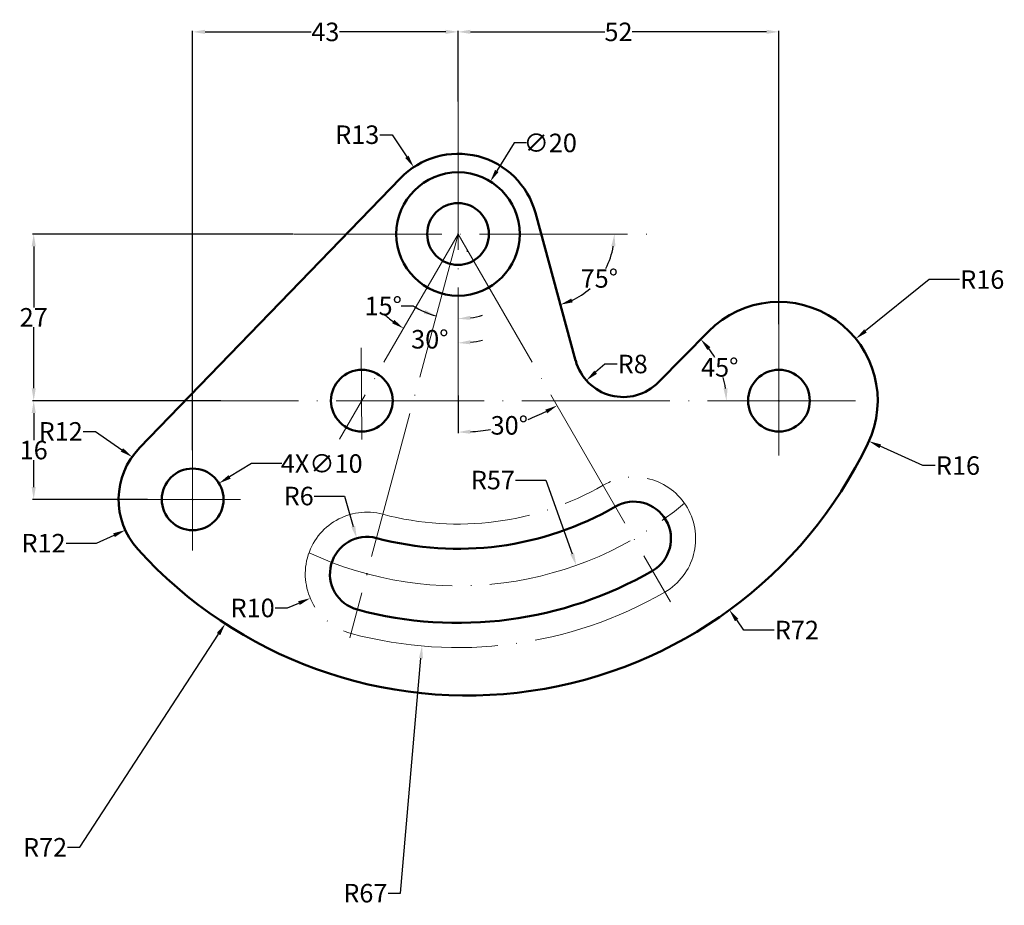
# Model space of a CAD drawing. Units: inches. Extents: x 244 to 404, y 121 to 265.
import ezdxf

# ---------------------------------------------------------------- set-up
doc = ezdxf.new("R2010")
doc.units = ezdxf.units.IN
doc.header["$MEASUREMENT"] = 0
doc.linetypes.add('ACAD_ISO04W100', pattern=[30, 24, -3, 0, -3])
for name, color, linetype, lineweight in [('M-CNTR', 4, 'ACAD_ISO04W100', 18), ('M-CONS', 4, 'ACAD_ISO04W100', 18), ('M-DIMS', 2, 'Continuous', 25), ('M-OUTL', 7, 'Continuous', 50)]:
    doc.layers.add(name, color=color, linetype=linetype, lineweight=lineweight)
doc.styles.get("Standard").update_dxf_attribs({"font": 'arial.ttf'})
doc.dimstyles.get("Standard").update_dxf_attribs({"dimtxt": 3, "dimasz": 2, "dimexe": 0.18, "dimexo": 0.0625, "dimgap": 0.09, "dimtad": 0, "dimtih": 1, "dimtoh": 1, "dimdec": 0, "dimzin": 0, "dimdsep": 46, "dimtxsty": 'Standard', "dimcen": 0.09, "dimadec": 0, "dimazin": 0, "dimtfac": 1, "dimtdec": 0, "dimtofl": 0, "dimtmove": 0, "dimatfit": 3, "dimfxl": 1, "dimtolj": 1, "dimtzin": 0, "dimarcsym": 0})

# ---------------------------------------------------------------- blocks, each defined once
blk = doc.blocks.new('*D1')
at = {"layer": 'Defpoints', "color": 0, "transparency": 16777216}
for p in [(316.73, 227.26), (359.19, 169.11)]:
    blk.add_point(p, dxfattribs=at)
at = {"layer": 'M-DIMS', "color": 0, "lineweight": -2, "transparency": 16777216}
for p, q in [((316.64, 227.26), (316.82, 227.26)), ((316.73, 227.17), (316.73, 227.35)), ((361.55, 165.87), (360.37, 167.5)), ((366.47, 165.87), (361.55, 165.87))]:
    blk.add_line(p, q, dxfattribs=at)
at = {"layer": 'M-DIMS', "color": 0, "transparency": 16777216}
blk.add_solid([(360.64, 167.69), (360.1, 167.3), (359.19, 169.11)], dxfattribs=at)
at = {"layer": 'M-DIMS', "color": 0, "transparency": 16777216, "insert": (370.13, 165.87), "char_height": 3, "attachment_point": 5}
blk.add_mtext('\\A1;R72', dxfattribs=at)
blk = doc.blocks.new('*D2')
at = {"layer": 'Defpoints', "color": 0, "transparency": 16777216}
for p in [(315.22, 230.03), (334.38, 176.35)]:
    blk.add_point(p, dxfattribs=at)
at = {"layer": 'M-DIMS', "color": 0, "lineweight": -2, "transparency": 16777216}
for p, q in [((324.54, 190.17), (329.45, 190.17)), ((329.45, 190.17), (333.71, 178.23))]:
    blk.add_line(p, q, dxfattribs=at)
at = {"layer": 'M-DIMS', "color": 0, "transparency": 16777216}
blk.add_solid([(334.02, 178.35), (333.4, 178.12), (334.38, 176.35)], dxfattribs=at)
at = {"layer": 'M-DIMS', "color": 0, "transparency": 16777216, "insert": (320.87, 190.17), "char_height": 3, "attachment_point": 5}
blk.add_mtext('\\A1;R57', dxfattribs=at)
blk = doc.blocks.new('*D3')
at = {"layer": 'Defpoints', "color": 0, "transparency": 16777216}
for p in [(300.47, 174.97), (291.28, 171.03)]:
    blk.add_point(p, dxfattribs=at)
at = {"layer": 'M-DIMS', "color": 0, "lineweight": -2, "transparency": 16777216}
for p, q in [((300.38, 174.97), (300.56, 174.97)), ((300.47, 174.88), (300.47, 175.06)), ((285.61, 169.45), (287.61, 169.45)), ((287.61, 169.45), (289.44, 170.24))]:
    blk.add_line(p, q, dxfattribs=at)
at = {"layer": 'M-DIMS', "color": 0, "transparency": 16777216}
blk.add_solid([(289.31, 170.54), (289.57, 169.93), (291.28, 171.03)], dxfattribs=at)
at = {"layer": 'M-DIMS', "color": 0, "transparency": 16777216, "insert": (281.94, 169.45), "char_height": 3, "attachment_point": 5}
blk.add_mtext('\\A1;R10', dxfattribs=at)
blk = doc.blocks.new('*D4')
at = {"layer": 'Defpoints', "color": 0, "transparency": 16777216}
for p in [(298.8, 180.74), (300.47, 174.97)]:
    blk.add_point(p, dxfattribs=at)
at = {"layer": 'M-DIMS', "color": 0, "lineweight": -2, "transparency": 16777216}
for p, q in [((291.91, 187.58), (296.81, 187.58)), ((296.81, 187.58), (298.24, 182.66)), ((300.38, 174.97), (300.56, 174.97)), ((300.47, 174.88), (300.47, 175.06))]:
    blk.add_line(p, q, dxfattribs=at)
at = {"layer": 'M-DIMS', "color": 0, "transparency": 16777216}
blk.add_solid([(298.56, 182.75), (297.92, 182.57), (298.8, 180.74)], dxfattribs=at)
at = {"layer": 'M-DIMS', "color": 0, "transparency": 16777216, "insert": (289.4, 187.58), "char_height": 3, "attachment_point": 5}
blk.add_mtext('\\A1;R6', dxfattribs=at)
blk = doc.blocks.new('*D5')
at = {"layer": 'Defpoints', "color": 0, "transparency": 16777216}
for p in [(272.22, 187.03), (261.3, 182.06)]:
    blk.add_point(p, dxfattribs=at)
at = {"layer": 'M-DIMS', "color": 0, "lineweight": -2, "transparency": 16777216}
for p, q in [((272.13, 187.03), (272.31, 187.03)), ((272.22, 186.94), (272.22, 187.12)), ((256.64, 179.94), (259.48, 181.23)), ((251.72, 179.94), (256.64, 179.94))]:
    blk.add_line(p, q, dxfattribs=at)
at = {"layer": 'M-DIMS', "color": 0, "transparency": 16777216}
blk.add_solid([(259.34, 181.54), (259.62, 180.93), (261.3, 182.06)], dxfattribs=at)
at = {"layer": 'M-DIMS', "color": 0, "transparency": 16777216, "insert": (248.06, 179.94), "char_height": 3, "attachment_point": 5}
blk.add_mtext('\\A1;R12', dxfattribs=at)
blk = doc.blocks.new('*D6')
at = {"layer": 'Defpoints', "color": 0, "transparency": 16777216}
for p in [(276.49, 189.64), (267.95, 184.43)]:
    blk.add_point(p, dxfattribs=at)
at = {"layer": 'M-DIMS', "color": 0, "lineweight": -2, "transparency": 16777216}
for p, q in [((281.73, 192.84), (278.2, 190.68)), ((286.65, 192.84), (281.73, 192.84)), ((272.13, 187.03), (272.31, 187.03)), ((272.22, 186.94), (272.22, 187.12))]:
    blk.add_line(p, q, dxfattribs=at)
at = {"layer": 'M-DIMS', "color": 0, "transparency": 16777216}
blk.add_solid([(278.02, 190.96), (278.37, 190.39), (276.49, 189.64)], dxfattribs=at)
at = {"layer": 'M-DIMS', "color": 0, "transparency": 16777216, "insert": (293.13, 192.84), "char_height": 3, "attachment_point": 5}
blk.add_mtext('\\A1;4X∅10', dxfattribs=at)
blk = doc.blocks.new('*D7')
at = {"layer": 'Defpoints', "color": 0, "transparency": 16777216}
for p in [(246.46, 203.03), (276.82, 203.03), (264.96, 187.03)]:
    blk.add_point(p, dxfattribs=at)
at = {"layer": 'M-DIMS', "color": 0, "lineweight": -2, "transparency": 16777216}
for p, q in [((276.76, 203.03), (246.28, 203.03)), ((246.46, 201.03), (246.46, 196.65)), ((246.46, 189.03), (246.46, 193.41)), ((264.89, 187.03), (246.28, 187.03))]:
    blk.add_line(p, q, dxfattribs=at)
at = {"layer": 'M-DIMS', "color": 0, "transparency": 16777216}
for points in [[(246.13, 201.03), (246.8, 201.03), (246.46, 203.03)], [(246.13, 189.03), (246.8, 189.03), (246.46, 187.03)]]:
    blk.add_solid(points, dxfattribs=at)
at = {"layer": 'M-DIMS', "color": 0, "transparency": 16777216, "insert": (246.46, 195.03), "char_height": 3, "attachment_point": 5}
blk.add_mtext('\\A1;16', dxfattribs=at)
blk = doc.blocks.new('*D8')
at = {"layer": 'Defpoints', "color": 0, "transparency": 16777216}
for p in [(246.46, 230.03), (288.6, 230.03), (276.82, 203.03)]:
    blk.add_point(p, dxfattribs=at)
at = {"layer": 'M-DIMS', "color": 0, "lineweight": -2, "transparency": 16777216}
for p, q in [((288.53, 230.03), (246.28, 230.03)), ((246.46, 228.03), (246.46, 218.13)), ((246.46, 205.03), (246.46, 214.94)), ((276.76, 203.03), (246.28, 203.03))]:
    blk.add_line(p, q, dxfattribs=at)
at = {"layer": 'M-DIMS', "color": 0, "transparency": 16777216}
for points in [[(246.13, 228.03), (246.8, 228.03), (246.46, 230.03)], [(246.13, 205.03), (246.8, 205.03), (246.46, 203.03)]]:
    blk.add_solid(points, dxfattribs=at)
at = {"layer": 'M-DIMS', "color": 0, "transparency": 16777216, "insert": (246.46, 216.53), "char_height": 3, "attachment_point": 5}
blk.add_mtext('\\A1;27', dxfattribs=at)
blk = doc.blocks.new('*D9')
at = {"layer": 'Defpoints', "color": 0, "transparency": 16777216}
for p in [(315.22, 262.78), (315.22, 251.46), (272.22, 194.96)]:
    blk.add_point(p, dxfattribs=at)
at = {"layer": 'M-DIMS', "color": 0, "lineweight": -2, "transparency": 16777216}
for p, q in [((272.22, 195.02), (272.22, 262.96)), ((274.22, 262.78), (291.42, 262.78)), ((313.22, 262.78), (296.02, 262.78)), ((315.22, 251.52), (315.22, 262.96))]:
    blk.add_line(p, q, dxfattribs=at)
at = {"layer": 'M-DIMS', "color": 0, "transparency": 16777216}
for points in [[(274.22, 263.12), (274.22, 262.45), (272.22, 262.78)], [(313.22, 263.12), (313.22, 262.45), (315.22, 262.78)]]:
    blk.add_solid(points, dxfattribs=at)
at = {"layer": 'M-DIMS', "color": 0, "transparency": 16777216, "insert": (293.72, 262.78), "char_height": 3, "attachment_point": 5}
blk.add_mtext('\\A1;43', dxfattribs=at)
blk = doc.blocks.new('*D10')
at = {"layer": 'Defpoints', "color": 0, "transparency": 16777216}
for p in [(367.22, 262.78), (315.22, 251.46), (367.22, 215.36)]:
    blk.add_point(p, dxfattribs=at)
at = {"layer": 'M-DIMS', "color": 0, "lineweight": -2, "transparency": 16777216}
for p, q in [((315.22, 251.52), (315.22, 262.96)), ((317.22, 262.78), (339, 262.78)), ((365.22, 262.78), (343.44, 262.78)), ((367.22, 215.43), (367.22, 262.96))]:
    blk.add_line(p, q, dxfattribs=at)
at = {"layer": 'M-DIMS', "color": 0, "transparency": 16777216}
for points in [[(317.22, 263.12), (317.22, 262.45), (315.22, 262.78)], [(365.22, 263.12), (365.22, 262.45), (367.22, 262.78)]]:
    blk.add_solid(points, dxfattribs=at)
at = {"layer": 'M-DIMS', "color": 0, "transparency": 16777216, "insert": (341.22, 262.78), "char_height": 3, "attachment_point": 5}
blk.add_mtext('\\A1;52', dxfattribs=at)
blk = doc.blocks.new('*D11')
at = {"layer": 'Defpoints', "color": 0, "transparency": 16777216}
for p in [(379.68, 213.07), (367.22, 203.03)]:
    blk.add_point(p, dxfattribs=at)
at = {"layer": 'M-DIMS', "color": 0, "lineweight": -2, "transparency": 16777216}
for p, q in [((391.58, 222.65), (381.24, 214.32)), ((396.49, 222.65), (391.58, 222.65)), ((367.13, 203.03), (367.31, 203.03)), ((367.22, 202.94), (367.22, 203.12))]:
    blk.add_line(p, q, dxfattribs=at)
at = {"layer": 'M-DIMS', "color": 0, "transparency": 16777216}
blk.add_solid([(381.03, 214.58), (381.45, 214.06), (379.68, 213.07)], dxfattribs=at)
at = {"layer": 'M-DIMS', "color": 0, "transparency": 16777216, "insert": (400.17, 222.65), "char_height": 3, "attachment_point": 5}
blk.add_mtext('\\A1;R16', dxfattribs=at)
blk = doc.blocks.new('*D12')
at = {"layer": 'Defpoints', "color": 0, "transparency": 16777216}
for p in [(315.22, 251.46), (315.22, 230.03), (314.02, 216.35), (315.22, 203.92), (297.69, 164.61)]:
    blk.add_point(p, dxfattribs=at)
at = {"layer": 'M-DIMS', "color": 0, "lineweight": -2, "transparency": 16777216}
blk.add_line((308, 218.36), (306, 218.36), dxfattribs=at)
for start, end in [(238.2486, 255), (238.2934, 246.6467), (278.3533, 286.7066)]:
    blk.add_arc((315.22, 230.03), 13.73, start, end, dxfattribs=at)
at = {"layer": 'M-DIMS', "color": 0, "transparency": 16777216}
for points in [[(309.89, 217.74), (309.67, 217.11), (311.67, 216.77)], [(317.24, 216.12), (317.19, 216.78), (315.22, 216.3)]]:
    blk.add_solid(points, dxfattribs=at)
at = {"layer": 'M-DIMS', "color": 0, "transparency": 16777216, "insert": (303.1, 218.36), "char_height": 3, "attachment_point": 5}
blk.add_mtext('\\A1;15°', dxfattribs=at)
blk = doc.blocks.new('*D13')
at = {"layer": 'Defpoints', "color": 0, "transparency": 16777216}
for p in [(315.22, 251.46), (315.22, 230.03), (315.22, 203.92), (320.79, 198.42), (349.63, 170.43)]:
    blk.add_point(p, dxfattribs=at)
at = {"layer": 'M-DIMS', "color": 0, "lineweight": -2, "transparency": 16777216}
blk.add_line((315.22, 203.86), (315.22, 197.75), dxfattribs=at)
for start, end in [(290.6871, 296.4296), (273.5704, 279.4609)]:
    blk.add_arc((315.22, 230.03), 32.1, start, end, dxfattribs=at)
at = {"layer": 'M-DIMS', "color": 0, "transparency": 16777216}
for points in [[(329.35, 201.58), (329.67, 200.99), (331.27, 202.23)], [(317.23, 197.66), (317.21, 198.33), (315.22, 197.93)]]:
    blk.add_solid(points, dxfattribs=at)
at = {"layer": 'M-DIMS', "color": 0, "transparency": 16777216, "insert": (323.53, 199.03), "char_height": 3, "attachment_point": 5}
blk.add_mtext('\\A1;30°', dxfattribs=at)
blk = doc.blocks.new('*D14')
at = {"layer": 'Defpoints', "color": 0, "transparency": 16777216}
for p in [(315.22, 251.46), (315.22, 230.03), (309.18, 213.44), (315.22, 203.92), (296.03, 196.79)]:
    blk.add_point(p, dxfattribs=at)
at = {"layer": 'M-DIMS', "color": 0, "lineweight": -2, "transparency": 16777216}
for start, end in [(227.0117, 233.5059), (276.4941, 282.9883)]:
    blk.add_arc((315.22, 230.03), 17.65, start, end, dxfattribs=at)
at = {"layer": 'M-DIMS', "color": 0, "transparency": 16777216}
for points in [[(304.9, 216.12), (304.54, 215.56), (306.39, 214.74)], [(317.24, 212.16), (317.2, 212.82), (315.22, 212.38)]]:
    blk.add_solid(points, dxfattribs=at)
at = {"layer": 'M-DIMS', "color": 0, "transparency": 16777216, "insert": (310.65, 212.98), "char_height": 3, "attachment_point": 5}
blk.add_mtext('\\A1;30°', dxfattribs=at)
blk = doc.blocks.new('*D15')
at = {"layer": 'Defpoints', "color": 0, "transparency": 16777216}
for p in [(327.76, 233.45), (288.6, 230.03), (348.27, 230.03), (336.34, 220.96), (334.28, 209.52)]:
    blk.add_point(p, dxfattribs=at)
at = {"layer": 'M-DIMS', "color": 0, "lineweight": -2, "transparency": 16777216}
for start, end in [(331.9016, 350.3305), (294.9017, 311.9853)]:
    blk.add_arc((328.69, 230.03), 11.86, start, end, dxfattribs=at)
at = {"layer": 'M-DIMS', "color": 0, "transparency": 16777216}
for points in [[(340.06, 228.07), (340.72, 228.01), (340.56, 230.03)], [(333.8, 218.96), (333.58, 219.58), (331.81, 218.58)]]:
    blk.add_solid(points, dxfattribs=at)
at = {"layer": 'M-DIMS', "color": 0, "transparency": 16777216, "insert": (338.12, 222.83), "char_height": 3, "attachment_point": 5}
blk.add_mtext('\\A1;75°', dxfattribs=at)
blk = doc.blocks.new('*D16')
at = {"layer": 'Defpoints', "color": 0, "transparency": 16777216}
for p in [(355.82, 214.26), (347.7, 206.01), (358.23, 206.68), (276.82, 203.03), (379.65, 203.03)]:
    blk.add_point(p, dxfattribs=at)
at = {"layer": 'M-DIMS', "color": 0, "lineweight": -2, "transparency": 16777216}
for start, end in [(30.1371, 37.2145), (8.2244, 15.6861)]:
    blk.add_arc((344.76, 203.03), 13.95, start, end, dxfattribs=at)
at = {"layer": 'M-DIMS', "color": 0, "transparency": 16777216}
for points in [[(355.62, 211.25), (356.12, 211.69), (354.55, 212.97)], [(358.9, 205.05), (358.23, 205), (358.71, 203.03)]]:
    blk.add_solid(points, dxfattribs=at)
at = {"layer": 'M-DIMS', "color": 0, "transparency": 16777216, "insert": (357.63, 208.42), "char_height": 3, "attachment_point": 5}
blk.add_mtext('\\A1;45°', dxfattribs=at)
blk = doc.blocks.new('*D17')
at = {"layer": 'Defpoints', "color": 0, "transparency": 16777216}
for p in [(342, 211.62), (336.02, 206.31)]:
    blk.add_point(p, dxfattribs=at)
at = {"layer": 'M-DIMS', "color": 0, "lineweight": -2, "transparency": 16777216}
for p, q in [((339.01, 208.97), (337.51, 207.64)), ((341.01, 208.97), (339.01, 208.97))]:
    blk.add_line(p, q, dxfattribs=at)
at = {"layer": 'M-DIMS', "color": 0, "transparency": 16777216}
blk.add_solid([(337.29, 207.89), (337.74, 207.39), (336.02, 206.31)], dxfattribs=at)
at = {"layer": 'M-DIMS', "color": 0, "transparency": 16777216, "insert": (343.52, 208.97), "char_height": 3, "attachment_point": 5}
blk.add_mtext('\\A1;R8', dxfattribs=at)
blk = doc.blocks.new('*D18')
at = {"layer": 'Defpoints', "color": 0, "transparency": 16777216}
for p in [(320.46, 238.55), (309.98, 221.51)]:
    blk.add_point(p, dxfattribs=at)
at = {"layer": 'M-DIMS', "color": 0, "lineweight": -2, "transparency": 16777216}
for p, q in [((324.29, 244.79), (321.51, 240.26)), ((326.29, 244.79), (324.29, 244.79)), ((315.13, 230.03), (315.31, 230.03)), ((315.22, 229.94), (315.22, 230.12))]:
    blk.add_line(p, q, dxfattribs=at)
at = {"layer": 'M-DIMS', "color": 0, "transparency": 16777216}
blk.add_solid([(321.22, 240.43), (321.79, 240.08), (320.46, 238.55)], dxfattribs=at)
at = {"layer": 'M-DIMS', "color": 0, "transparency": 16777216, "insert": (330.16, 244.79), "char_height": 3, "attachment_point": 5}
blk.add_mtext('\\A1;∅20', dxfattribs=at)
blk = doc.blocks.new('*D19')
at = {"layer": 'Defpoints', "color": 0, "transparency": 16777216}
for p in [(308.04, 240.87), (315.22, 230.03)]:
    blk.add_point(p, dxfattribs=at)
at = {"layer": 'M-DIMS', "color": 0, "lineweight": -2, "transparency": 16777216}
for p, q in [((302.56, 246.12), (304.56, 246.12)), ((304.56, 246.12), (306.94, 242.54)), ((315.13, 230.03), (315.31, 230.03)), ((315.22, 229.94), (315.22, 230.12))]:
    blk.add_line(p, q, dxfattribs=at)
at = {"layer": 'M-DIMS', "color": 0, "transparency": 16777216}
blk.add_solid([(307.21, 242.72), (306.66, 242.35), (308.04, 240.87)], dxfattribs=at)
at = {"layer": 'M-DIMS', "color": 0, "transparency": 16777216, "insert": (298.89, 246.12), "char_height": 3, "attachment_point": 5}
blk.add_mtext('\\A1;R13', dxfattribs=at)
blk = doc.blocks.new('POSITION-HOLE-D10')
blk.add_circle((5, 5), 5)
blk = doc.blocks.new('*D21')
at = {"layer": 'Defpoints', "color": 0, "transparency": 16777216}
for p in [(262.39, 193.92), (272.22, 187.03)]:
    blk.add_point(p, dxfattribs=at)
at = {"layer": 'M-DIMS', "color": 0, "lineweight": -2, "transparency": 16777216}
for p, q in [((254.5, 198.05), (256.5, 198.05)), ((256.5, 198.05), (260.75, 195.07)), ((272.13, 187.03), (272.31, 187.03)), ((272.22, 186.94), (272.22, 187.12))]:
    blk.add_line(p, q, dxfattribs=at)
at = {"layer": 'M-DIMS', "color": 0, "transparency": 16777216}
blk.add_solid([(260.95, 195.34), (260.56, 194.79), (262.39, 193.92)], dxfattribs=at)
at = {"layer": 'M-DIMS', "color": 0, "transparency": 16777216, "insert": (250.84, 198.05), "char_height": 3, "attachment_point": 5}
blk.add_mtext('\\A1;R12', dxfattribs=at)
blk = doc.blocks.new('*D22')
at = {"layer": 'Defpoints', "color": 0, "transparency": 16777216}
for p in [(367.22, 203.03), (381.81, 196.46)]:
    blk.add_point(p, dxfattribs=at)
at = {"layer": 'M-DIMS', "color": 0, "lineweight": -2, "transparency": 16777216}
for p, q in [((367.13, 203.03), (367.31, 203.03)), ((367.22, 202.94), (367.22, 203.12)), ((390.56, 192.52), (383.63, 195.64)), ((392.56, 192.52), (390.56, 192.52))]:
    blk.add_line(p, q, dxfattribs=at)
at = {"layer": 'M-DIMS', "color": 0, "transparency": 16777216}
blk.add_solid([(383.77, 195.94), (383.5, 195.34), (381.81, 196.46)], dxfattribs=at)
at = {"layer": 'M-DIMS', "color": 0, "transparency": 16777216, "insert": (396.23, 192.52), "char_height": 3, "attachment_point": 5}
blk.add_mtext('\\A1;R16', dxfattribs=at)
blk = doc.blocks.new('*D23')
at = {"layer": 'Defpoints', "color": 0, "transparency": 16777216}
for p in [(316.73, 227.26), (277.5, 166.89)]:
    blk.add_point(p, dxfattribs=at)
at = {"layer": 'M-DIMS', "color": 0, "lineweight": -2, "transparency": 16777216}
for p, q in [((316.64, 227.26), (316.82, 227.26)), ((316.73, 227.17), (316.73, 227.35)), ((253.96, 130.67), (276.41, 165.21)), ((251.96, 130.67), (253.96, 130.67))]:
    blk.add_line(p, q, dxfattribs=at)
at = {"layer": 'M-DIMS', "color": 0, "transparency": 16777216}
blk.add_solid([(276.13, 165.4), (276.69, 165.03), (277.5, 166.89)], dxfattribs=at)
at = {"layer": 'M-DIMS', "color": 0, "transparency": 16777216, "insert": (248.3, 130.67), "char_height": 3, "attachment_point": 5}
blk.add_mtext('\\A1;R72', dxfattribs=at)
blk = doc.blocks.new('*D24')
at = {"layer": 'Defpoints', "color": 0, "transparency": 16777216}
for p in [(315.22, 230.03), (309.38, 163.29)]:
    blk.add_point(p, dxfattribs=at)
at = {"layer": 'M-DIMS', "color": 0, "lineweight": -2, "transparency": 16777216}
for p, q in [((315.13, 230.03), (315.31, 230.03)), ((315.22, 229.94), (315.22, 230.12)), ((305.88, 123.24), (309.21, 161.3)), ((303.88, 123.24), (305.88, 123.24))]:
    blk.add_line(p, q, dxfattribs=at)
at = {"layer": 'M-DIMS', "color": 0, "transparency": 16777216}
blk.add_solid([(308.87, 161.32), (309.54, 161.27), (309.38, 163.29)], dxfattribs=at)
at = {"layer": 'M-DIMS', "color": 0, "transparency": 16777216, "insert": (300.2, 123.24), "char_height": 3, "attachment_point": 5}
blk.add_mtext('\\A1;R67', dxfattribs=at)

msp = doc.modelspace()

# ---------------------------------------------------------------- linework, layer by layer
at = {"layer": 'M-CNTR'}
for p, q in [((315.22, 251.46), (315.22, 203.92)), ((288.6, 230.03), (348.27, 230.03)), ((315.22, 230.03), (296.03, 196.79)), ((315.22, 230.03), (297.69, 164.61)), ((315.22, 230.03), (349.63, 170.43)), ((367.22, 194.14), (367.22, 215.36)), ((299.63, 196.73), (299.54, 211.6)), ((379.65, 203.03), (276.82, 203.03)), ((272.22, 178.74), (272.22, 194.96)), ((264.96, 187.03), (279.98, 187.03))]:
    msp.add_line(p, q, dxfattribs=at)
msp.add_arc((315.22, 230.03), 57, 244.9352, 310.0648, dxfattribs=at)
at = {"layer": 'M-CONS'}
for centre, radius, start, end in [((343.72, 180.67), 10, 300, 120), ((315.22, 230.03), 47, 255, 300), ((300.47, 174.97), 10, 75, 255), ((315.22, 230.03), 67, 255, 300)]:
    msp.add_arc(centre, radius, start, end, dxfattribs=at)
at = {"layer": 'M-OUTL'}
for p, q in [((263.6, 195.38), (305.88, 239.07)), ((327.76, 233.45), (334.28, 209.52)), ((355.82, 214.26), (347.7, 206.01))]:
    msp.add_line(p, q, dxfattribs=at)
msp.add_circle((315.22, 230.03), 10, dxfattribs=at)
for centre, radius, start, end in [((315.22, 230.03), 13, 15.2322, 135.9422), ((367.22, 203.03), 16, 334.3613, 135.4388), ((342, 211.62), 8, 195.2322, 315.4388), ((272.22, 187.03), 12, 135.9422, 222.1069), ((316.73, 227.26), 72, 222.1069, 334.3613), ((343.72, 180.67), 6, 300, 120), ((315.22, 230.03), 51, 255, 300), ((300.47, 174.97), 6, 75, 255), ((315.22, 230.03), 63, 255, 300)]:
    msp.add_arc(centre, radius, start, end, dxfattribs=at)

# ---------------------------------------------------------------- block references
for p in [(310.22, 225.03), (294.63, 198.03), (362.22, 198.03), (267.22, 182.03)]:
    msp.add_blockref('POSITION-HOLE-D10', p, dxfattribs=at)

# ---------------------------------------------------------------- dimensions: what is measured, and where the dimension line sits
at = {"layer": 'M-DIMS'}
for base, p1, p2, picture, middle in [((315.22, 262.78), (272.22, 194.96), (315.22, 251.46), '*D9', (293.72, 262.78)), ((367.22, 262.78), (315.22, 251.46), (367.22, 215.36), '*D10', (341.22, 262.78))]:
    dim = msp.add_linear_dim(base=base, p1=p1, p2=p2, dimstyle='Standard', override={"dimclrd": 0, "dimclre": 0, "dimclrt": 0}, dxfattribs=at)
    dim.commit()
    dim.dimension.update_dxf_attribs({"geometry": picture, "text_midpoint": middle})
for base, line1, line2, picture, middle in [((309.18, 213.44), ((315.22, 230.03), (296.03, 196.79)), ((315.22, 251.46), (315.22, 203.92)), '*D14', (310.65, 212.98)), ((314.02, 216.35), ((315.22, 251.46), (315.22, 203.92)), ((315.22, 230.03), (297.69, 164.61)), '*D12', (303.1, 218.36)), ((320.79, 198.42), ((315.22, 230.03), (349.63, 170.43)), ((315.22, 251.46), (315.22, 203.92)), '*D13', (323.53, 199.03)), ((336.34, 220.96), ((327.76, 233.45), (334.28, 209.52)), ((288.6, 230.03), (348.27, 230.03)), '*D15', (338.12, 222.83)), ((358.23, 206.68), ((379.65, 203.03), (276.82, 203.03)), ((355.82, 214.26), (347.7, 206.01)), '*D16', (357.63, 208.42))]:
    dim = msp.add_angular_dim_2l(base=base, line1=line1, line2=line2, dimstyle='Standard', override={"dimclrd": 0, "dimclre": 0, "dimclrt": 0}, dxfattribs=at)
    dim.commit()
    dim.dimension.update_dxf_attribs({"geometry": picture, "text_midpoint": middle})
for center, mpoint, override, picture, middle in [((315.22, 230.03), (308.04, 240.87), {"dimclrd": 0, "dimclre": 0, "dimclrt": 0}, '*D19', (298.89, 246.12)), ((315.22, 230.03), (309.38, 163.29), {"dimdec": 0, "dimlfac": 1, "dimrnd": 0, "dimzin": 0, "dimdsep": 46, "dimlunit": 2}, '*D24', (300.2, 123.24)), ((315.22, 230.03), (334.38, 176.35), {"dimclrd": 0, "dimclre": 0, "dimclrt": 0}, '*D2', (320.87, 190.17)), ((316.73, 227.26), (277.5, 166.89), {"dimdec": 0, "dimlfac": 1, "dimrnd": 0, "dimzin": 0, "dimdsep": 46, "dimlunit": 2}, '*D23', (248.3, 130.67)), ((316.73, 227.26), (359.19, 169.11), {"dimclrd": 0, "dimclre": 0, "dimclrt": 0}, '*D1', (370.13, 165.87)), ((367.22, 203.03), (379.68, 213.07), {"dimclrd": 0, "dimclre": 0, "dimclrt": 0}, '*D11', (400.17, 222.65)), ((342, 211.62), (336.02, 206.31), {"dimclrd": 0, "dimclre": 0, "dimclrt": 0}, '*D17', (343.52, 208.97)), ((367.22, 203.03), (381.81, 196.46), {"dimdec": 0, "dimlfac": 1, "dimrnd": 0, "dimzin": 0, "dimdsep": 46, "dimlunit": 2}, '*D22', (396.23, 192.52)), ((272.22, 187.03), (262.39, 193.92), {"dimdec": 0, "dimlfac": 1, "dimrnd": 0, "dimzin": 0, "dimdsep": 46, "dimlunit": 2}, '*D21', (250.84, 198.05)), ((300.47, 174.97), (298.8, 180.74), {"dimclrd": 0, "dimclre": 0, "dimclrt": 0}, '*D4', (289.4, 187.58)), ((272.22, 187.03), (261.3, 182.06), {"dimclrd": 0, "dimclre": 0, "dimclrt": 0}, '*D5', (248.06, 179.94))]:
    dim = msp.add_radius_dim(center=center, mpoint=mpoint, dimstyle='Standard', override=override, dxfattribs=at)
    dim.commit()
    dim.dimension.update_dxf_attribs({"geometry": picture, "text_midpoint": middle, "dimtype": 164})
dim = msp.add_diameter_dim_2p(p1=(309.98, 221.51), p2=(320.46, 238.55), dimstyle='Standard', override={"dimclrd": 0, "dimclre": 0, "dimclrt": 0}, dxfattribs=at)
dim.commit()
dim.dimension.update_dxf_attribs({"geometry": '*D18', "text_midpoint": (330.16, 244.79), "dimtype": 163})
for base, p1, p2, picture, middle in [((246.46, 230.03), (276.82, 203.03), (288.6, 230.03), '*D8', (246.46, 216.53)), ((246.46, 203.03), (264.96, 187.03), (276.82, 203.03), '*D7', (246.46, 195.03))]:
    dim = msp.add_linear_dim(base=base, p1=p1, p2=p2, angle=90, dimstyle='Standard', override={"dimclrd": 0, "dimclre": 0, "dimclrt": 0}, dxfattribs=at)
    dim.commit()
    dim.dimension.update_dxf_attribs({"geometry": picture, "text_midpoint": middle})
dim = msp.add_diameter_dim_2p(p1=(267.95, 184.43), p2=(276.49, 189.64), text='4X<>', dimstyle='Standard', override={"dimclrd": 0, "dimclre": 0, "dimclrt": 0}, dxfattribs=at)
dim.commit()
dim.dimension.update_dxf_attribs({"geometry": '*D6', "text_midpoint": (293.13, 192.84), "dimtype": 163})
dim = msp.add_radius_dim(center=(300.47, 174.97), mpoint=(291.28, 171.03), dimstyle='Standard', override={"dimclrd": 0, "dimclre": 0, "dimclrt": 0}, dxfattribs=at)
dim.commit()
dim.dimension.update_dxf_attribs({"geometry": '*D3', "text_midpoint": (281.94, 169.45)})

doc.saveas('drawing.dxf')
